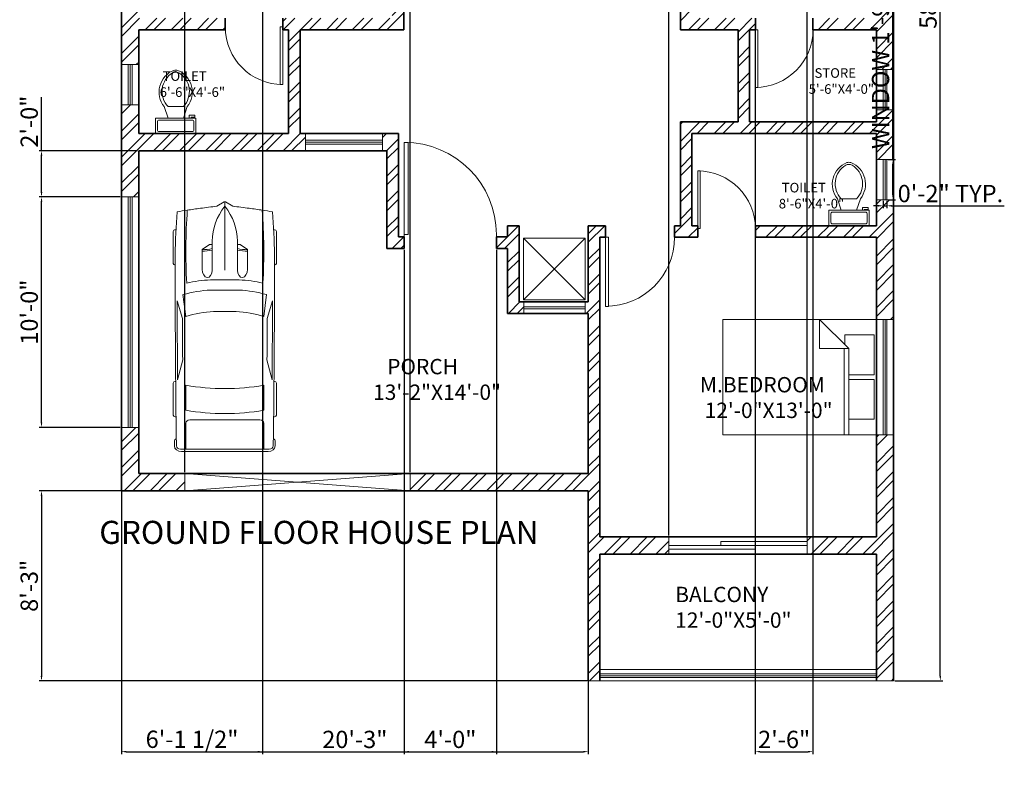
# Model space of a CAD drawing. Units: inches. Extents: x 73 to 724, y 1566 to 2355.
# Tile 1 of 2: x 147 to 660, y 1566 to 1955. Entities that reach past the tile are written whole.
import ezdxf

# ---------------------------------------------------------------- set-up
doc = ezdxf.new("R2010")
doc.units = ezdxf.units.IN
for name, color, linetype, lineweight in [('A-ANNO-DIMS', 2, 'Continuous', 18), ('A-ANNO-TEXT', 7, 'Continuous', 25), ('A-AREA-IDEN', 7, 'Continuous', 18), ('A-DOOR', 4, 'Continuous', 18), ('A-EQPM-VEHC', 8, 'Continuous', 13), ('A-FLOR', 7, 'Continuous', 18), ('A-FLOR-FIXT', 9, 'Continuous', 18), ('A-FLOR-RAIL', 244, 'Continuous', 18), ('A-FURN', 9, 'Continuous', 18), ('A-GLAZ', 244, 'Continuous', 18), ('A-WALL', 7, 'Continuous', 35), ('A-WALL-PATT', 252, 'Continuous', 13)]:
    doc.layers.add(name, color=color, linetype=linetype, lineweight=lineweight)
doc.styles.get("Standard").update_dxf_attribs({"font": 'arial.ttf'})
doc.dimstyles.new('ISO-25', dxfattribs={"dimtxt": 9, "dimasz": 2.5, "dimexe": 1.25, "dimexo": 0.625, "dimtad": 1, "dimlunit": 3, "dimtxsty": 'Standard', "dimcen": 2.5, "dimadec": 0, "dimazin": 0, "dimtfac": 1, "dimtmove": 0, "dimatfit": 3, "dimfxl": 1, "dimarcsym": 0})

# ---------------------------------------------------------------- blocks, each defined once
blk = doc.blocks.new('*U2')
for p, q in [((0, 0), (0, -6)), ((40, 0), (40, -6))]:
    blk.add_line(p, q)
blk.add_lwpolyline([(0, 0), (0, 40), (1.75, 40), (1.75, 0)], close=True)
blk.add_arc((0, 0), 40, 0, 90)
blk = doc.blocks.new('*U6')
for p, q in [((0, 0), (0, 6)), ((40, 0), (40, 6))]:
    blk.add_line(p, q)
blk.add_lwpolyline([(0, 0), (0, -40), (1.75, -40), (1.75, 0)], close=True)
blk.add_arc((0, 0), 40, 270, 0)
blk = doc.blocks.new('*U7')
for p, q in [((0, 0), (0, -6)), ((40, 0), (40, -6))]:
    blk.add_line(p, q)
blk.add_lwpolyline([(0, 0), (0, 40), (1.75, 40), (1.75, 0)], close=True)
blk.add_arc((0, 0), 40, 0, 90)
blk = doc.blocks.new('*U8')
for p, q in [((-40, 0), (-40, 6)), ((0, 0), (0, 6))]:
    blk.add_line(p, q)
blk.add_lwpolyline([(0, 0), (0, -40), (-1.75, -40), (-1.75, 0)], close=True)
blk.add_arc((0, 0), 40, 180, 270)
blk = doc.blocks.new('*D10')
at = {"layer": 'A-ANNO-DIMS', "color": 0, "lineweight": -2, "transparency": 16777216}
for p, q in [((602.66, 2307.12), (627.57, 2307.12)), ((626.32, 1613.62), (626.32, 2304.62)), ((602.66, 1611.12), (627.57, 1611.12))]:
    blk.add_line(p, q, dxfattribs=at)
at = {"layer": 'A-ANNO-DIMS', "color": 0, "transparency": 16777216}
for points in [[(625.9, 2304.62), (626.74, 2304.62), (626.32, 2307.12)], [(625.9, 1613.62), (626.74, 1613.62), (626.32, 1611.12)]]:
    blk.add_solid(points, dxfattribs=at)
at = {"layer": 'Defpoints', "color": 0, "transparency": 16777216}
for p in [(602.03, 2307.12), (626.32, 2307.12), (602.03, 1611.12)]:
    blk.add_point(p, dxfattribs=at)
at = {"layer": 'A-ANNO-DIMS', "color": 0, "transparency": 16777216, "insert": (621.1, 1959.12), "char_height": 9, "attachment_point": 5, "rotation": 90}
blk.add_mtext("58'", dxfattribs=at)
blk = doc.blocks.new('Bed - Queen')
for p, q in [((0, -80.00003), (0, 0)), ((0, 0), (59.99999, 0)), ((59.99999, 0), (59.99999, -80.00003)), ((7.99999, -1.2), (28.79998, -1.2)), ((7.99999, -14.4), (7.99999, -1.2)), ((28.79998, -1.2), (28.79998, -14.4)), ((31.19999, -1.2), (51.99999, -1.2)), ((31.19999, -14.4), (31.19999, -1.2)), ((51.99999, -1.2), (51.99999, -16.4)), ((0, -14.4), (44.8, -14.4)), ((59.99999, -29.6), (44.8, -14.4)), ((44.8, -14.4), (44.8, -29.6)), ((44.8, -16.8), (0, -16.8)), ((51.99999, -16.4), (46.79936, -16.4)), ((44.8, -29.6), (59.99999, -29.6)), ((59.99999, -80.00003), (0, -80.00003))]:
    blk.add_line(p, q)
blk = doc.blocks.new('*U13')
for p, q in [((9.5, -6), (9.5, -2)), ((-10, -8.5), (-8, -8.5)), ((-10, -9.5), (-10, -8.5)), ((-7, -9.5), (-10, -9.5)), ((-8, -8.5), (-8, -8)), ((-7, -8), (-7, -9.5)), ((-4, -8), (-6, -14)), ((4, -8), (6, -14)), ((4, -14), (-4, -14))]:
    blk.add_line(p, q)
blk.add_lwpolyline([(10.5, -8), (10.5, 0), (-10.5, 0), (-10.5, -8)], close=True)
for points in [[(-9.5, -2), (-9.5, -6)], [(8.5, -1), (-8.5, -1)], [(-8.5, -7), (8.5, -7)]]:
    blk.add_lwpolyline(points)
for centre, radius, start, end in [((-8.62, -1.88), 0.884, 81.8699, 188.1301), ((8.62, -1.88), 0.884, 351.8699, 98.1301), ((-8.62, -6.12), 0.884, 171.8699, 278.1301), ((8.62, -6.12), 0.884, 261.8699, 8.1301), ((3.52, -21.58), 12.17, 141.4691, 247.9714), ((4.2, -21.82), 11.33, 136.3677, 238.9468), ((-3.52, -21.58), 12.17, 292.0284, 38.5307), ((-4.2, -21.82), 11.33, 301.053, 43.6321), ((0, -27.88), 4, 245.7318, 294.2682), ((0, -29), 4, 254.8605, 285.1395)]:
    blk.add_arc(centre, radius, start, end)
blk = doc.blocks.new('*U15')
for p, q in [((21.1, 37.41), (21.1, 36.83)), ((46.55, 38.89), (22.35, 38.89)), ((47.8, 37.39), (47.8, 37.41)), ((135.45, 37.07), (135.45, 37.41)), ((136.7, 38.89), (160.9, 38.89)), ((162.15, 37.41), (162.15, 36.77)), ((70.03, 31.54), (86.41, 29.35)), ((87.99, 31.87), (74.76, 35.92)), ((134.31, 35.6), (119.29, 31.78)), ((186.47, -33.5), (186.47, 33.5)), ((188.4, -32.76), (188.4, 32.76)), ((138.42, 29.35), (157.25, 29.35)), ((164.52, 26.39), (164.52, -26.39)), ((186.47, 29.35), (167.01, 29.35)), ((32.27, 11.63), (36.13, 17.17)), ((36.13, 17.17), (50.94, 17.17)), ((29.77, 9.51), (51.68, 9.51)), ((32.12, 9.51), (32.12, 11.15)), ((58.92, -10.77), (58.92, 10.77)), ((66.55, -10.53), (66.55, 10.53)), ((82.74, 8.5), (82.74, -8.5)), ((186.47, -10.53), (186.47, 10.53)), ((3.27, 6.13), (0.1, 0.41)), ((0, 0), (51.68, 0)), ((0.1, -0.41), (3.27, -6.13)), ((29.77, -9.51), (51.68, -9.51)), ((32.12, -9.51), (32.12, -11.15)), ((32.27, -11.63), (36.13, -17.17)), ((36.13, -17.17), (50.94, -17.17)), ((86.41, -29.35), (70.03, -31.54)), ((157.25, -29.35), (138.42, -29.35)), ((167.01, -29.35), (186.47, -29.35)), ((21.1, -37.41), (21.1, -36.83)), ((87.99, -31.87), (74.76, -35.92)), ((134.31, -35.6), (119.29, -31.78)), ((135.45, -37.07), (135.45, -37.41)), ((162.15, -37.41), (162.15, -36.77)), ((46.55, -38.89), (22.35, -38.89)), ((47.8, -37.39), (47.8, -37.41)), ((136.7, -38.89), (160.9, -38.89))]:
    blk.add_line(p, q)
for centre, major_axis, ratio, start_param, end_param in [((41.19, -490.86), (0, 528.23), 0.842304, 0.00281, 0.075598), ((22.35, 37.41), (0, -1.48), 0.842304, 3.141593, 4.712389), ((64.48, -10555.62), (0, 10593.03), 0.842304, -0.013397, 0.002797), ((46.55, 37.41), (0, 1.48), 0.842304, -1.570796, 0), ((136.7, 37.41), (0, -1.48), 0.842304, 3.141593, 4.712389), ((160.9, 37.41), (0, 1.48), 0.842304, -1.570796, 0), ((180.63, 35.84), (0, 2.22), 0.842304, -0.013017, 1.249894), ((64.48, -10556.36), (0, 10595.31), 0.842304, -0.013397, -0.013017), ((183.98, 32.76), (0, -5.25), 0.842304, 1.570796, 3.128196), ((266.03, -27.52), (0, 313.31), 0.842304, 1.367076, 1.39176), ((37.47, -593.96), (0, -623.33), 0.842304, 3.096046, 3.200911), ((135.29, 5.39), (0, 81.77), 0.842304, 1.245306, 1.50788), ((64.48, -10555.62), (0, -10591.55), 0.842304, 3.133765, 3.140441), ((95.79, -3666.35), (0, -3698.24), 0.842304, 3.134049, 3.144098), ((183.98, 33.5), (0, -2.96), 0.842304, 1.570796, 3.128196), ((259.18, -27.52), (0, -305.3), 0.842304, 4.528606, 4.561838), ((134.4, 5.39), (0, -89.78), 0.842304, 4.449482, 4.652344), ((149.6, 2.8), (0, -79.58), 0.842304, 4.372215, 4.640744), ((17.08, 0), (0, 147.02), 0.842304, 4.511394, 4.913384), ((35.91, 0), (0, 147.02), 0.842304, 4.511394, 4.913384), ((167.01, 26.39), (0, 2.96), 0.842304, 0, 1.570796), ((-204.49, 52.4), (0, -250.96), 0.842304, 1.385369, 1.434372), ((13.04, 17.01), (0, 27.42), 0.842304, 4.435146, 4.718221), ((14.2, 17.01), (0, 27.42), 0.842304, 4.435146, 4.718221), ((50.79, 13.34), (6.34, -0.36), 0.603834, -1.395552, 1.581315), ((29.77, -46.66), (0, 56.17), 0.842304, 0, 0.590319), ((32.75, 11.15), (0, 0.74), 0.842304, 0.879714, 1.570796), ((0.62, 0), (0, -0.74), 0.842304, 4.131459, 5.293319), ((-204.49, -52.4), (0, 250.96), 0.842304, -1.434372, -1.385369), ((29.77, 46.66), (0, 56.17), 0.842304, 2.551274, 3.141593), ((32.75, -11.15), (0, -0.74), 0.842304, 4.712389, 5.403472), ((13.04, -17.01), (0, -27.42), 0.842304, 1.564964, 1.848039), ((14.2, -17.01), (0, -27.42), 0.842304, 1.564964, 1.848039), ((134.4, -5.39), (0, -89.78), 0.842304, -1.510751, -1.307889), ((135.29, -5.39), (0, -81.77), 0.842304, -1.50788, -1.245306), ((149.6, -2.8), (0, -79.58), 0.842304, -1.499151, -1.230623), ((259.18, 27.52), (0, 305.3), 0.842304, 1.721348, 1.754579), ((266.03, 27.52), (0, 313.31), 0.842304, 1.749832, 1.774517), ((37.47, 593.96), (0, -623.33), 0.842304, -0.059319, 0.045547), ((167.01, -26.39), (0, -2.96), 0.842304, 4.712389, 6.283185), ((41.19, 490.86), (0, -528.23), 0.842304, -0.075598, -0.00281), ((64.48, 10555.62), (0, 10593.03), 0.842304, 3.138796, 3.15499), ((64.48, 10555.62), (0, -10591.55), 0.842304, 0.001152, 0.007828), ((95.79, 3666.35), (0, -3698.24), 0.842304, -0.002505, 0.007544), ((180.63, -35.84), (0, -2.22), 0.842304, -1.249894, 0.013017), ((183.98, -33.5), (0, 2.96), 0.842304, 3.15499, 4.712389), ((183.98, -32.76), (0, -5.25), 0.842304, 0.013397, 1.570796), ((22.35, -37.41), (0, 1.48), 0.842304, 1.570796, 3.141593), ((46.55, -37.41), (0, -1.48), 0.842304, 0, 1.570796), ((136.7, -37.41), (0, -1.48), 0.842304, -1.570796, 0), ((160.9, -37.41), (0, 1.48), 0.842304, 3.141593, 4.712389), ((64.48, 10556.36), (0, 10595.31), 0.842304, 3.15461, 3.15499)]:
    blk.add_ellipse(centre, major_axis=major_axis, ratio=ratio, start_param=start_param, end_param=end_param)
at = {"extrusion": (0, 0, -1)}
blk.add_ellipse((50.79, -13.34), major_axis=(6.34, 0.36), ratio=0.603834, start_param=-1.395552, end_param=1.581315, dxfattribs=at)
blk = doc.blocks.new('WIN-GLAZING-60IN')
for p, q in [((0, 2), (60, 2)), ((0, 1), (60, 1)), ((0, 0), (60, 0))]:
    blk.add_line(p, q)
blk = doc.blocks.new('WIN-GLAZING-21IN')
for p, q in [((0, 21), (0, 0)), ((1, 21), (1, 0)), ((2, 21), (2, 0))]:
    blk.add_line(p, q)
blk = doc.blocks.new('*D21')
at = {"layer": 'A-ANNO-DIMS', "color": 0, "lineweight": -2, "transparency": 16777216}
for p, q in [((601.68, 1882.62), (601.68, 2000.26)), ((599.16, 1882.62), (602.93, 1882.62)), ((601.68, 1864.12), (601.68, 1880.12)), ((599.16, 1861.62), (602.93, 1861.62))]:
    blk.add_line(p, q, dxfattribs=at)
at = {"layer": 'A-ANNO-DIMS', "color": 0, "transparency": 16777216}
for points in [[(601.27, 1880.12), (602.1, 1880.12), (601.68, 1882.62)], [(601.27, 1864.12), (602.1, 1864.12), (601.68, 1861.62)]]:
    blk.add_solid(points, dxfattribs=at)
at = {"layer": 'Defpoints', "color": 0, "transparency": 16777216}
for p in [(598.53, 1882.62), (601.68, 1882.62), (598.53, 1861.62)]:
    blk.add_point(p, dxfattribs=at)
at = {"layer": 'A-ANNO-DIMS', "color": 0, "transparency": 16777216, "insert": (596.4, 1942.69), "char_height": 9, "attachment_point": 5, "rotation": 90}
blk.add_mtext('WINDOW 1\'-9" TYP.', dxfattribs=at)
blk = doc.blocks.new('*D22')
at = {"layer": 'A-ANNO-DIMS', "color": 0, "lineweight": -2, "transparency": 16777216}
for p, q in [((596.53, 1861), (596.53, 1857.22)), ((598.53, 1861), (598.53, 1857.22)), ((594.03, 1858.47), (591.53, 1858.47)), ((596.53, 1858.47), (598.53, 1858.47)), ((601.03, 1858.47), (659.64, 1858.47))]:
    blk.add_line(p, q, dxfattribs=at)
at = {"layer": 'A-ANNO-DIMS', "color": 0, "transparency": 16777216}
for points in [[(594.03, 1858.89), (594.03, 1858.06), (596.53, 1858.47)], [(601.03, 1858.89), (601.03, 1858.06), (598.53, 1858.47)]]:
    blk.add_solid(points, dxfattribs=at)
at = {"layer": 'Defpoints', "color": 0, "transparency": 16777216}
for p in [(596.53, 1861.62), (598.53, 1861.62), (598.53, 1858.47)]:
    blk.add_point(p, dxfattribs=at)
at = {"layer": 'A-ANNO-DIMS', "color": 0, "transparency": 16777216, "insert": (631.59, 1863.69), "char_height": 9, "attachment_point": 5}
blk.add_mtext('0\'-2" TYP.', dxfattribs=at)
blk = doc.blocks.new('*D27')
at = {"layer": 'A-ANNO-DIMS', "color": 0, "lineweight": -2, "transparency": 16777216}
for p, q in [((200.03, 1709.5), (200.03, 1573.02)), ((443.03, 1709.5), (443.03, 1573.02)), ((202.53, 1574.27), (440.53, 1574.27))]:
    blk.add_line(p, q, dxfattribs=at)
at = {"layer": 'A-ANNO-DIMS', "color": 0, "transparency": 16777216}
for points in [[(202.53, 1574.69), (202.53, 1573.86), (200.03, 1574.27)], [(440.53, 1574.69), (440.53, 1573.86), (443.03, 1574.27)]]:
    blk.add_solid(points, dxfattribs=at)
at = {"layer": 'Defpoints', "color": 0, "transparency": 16777216}
for p in [(200.03, 1710.12), (443.03, 1710.12), (443.03, 1574.27)]:
    blk.add_point(p, dxfattribs=at)
at = {"layer": 'A-ANNO-DIMS', "color": 0, "transparency": 16777216, "insert": (321.53, 1579.49), "char_height": 9, "attachment_point": 5}
blk.add_mtext('20\'-3"', dxfattribs=at)
blk = doc.blocks.new('*D28')
at = {"layer": 'A-ANNO-DIMS', "color": 0, "lineweight": -2, "transparency": 16777216}
for p, q in [((442.41, 1710.12), (157.17, 1710.12)), ((158.42, 1707.62), (158.42, 1613.62)), ((442.41, 1611.12), (157.17, 1611.12))]:
    blk.add_line(p, q, dxfattribs=at)
at = {"layer": 'A-ANNO-DIMS', "color": 0, "transparency": 16777216}
for points in [[(158, 1707.62), (158.84, 1707.62), (158.42, 1710.12)], [(158, 1613.62), (158.84, 1613.62), (158.42, 1611.12)]]:
    blk.add_solid(points, dxfattribs=at)
at = {"layer": 'Defpoints', "color": 0, "transparency": 16777216}
for p in [(443.03, 1710.12), (158.42, 1611.12), (443.03, 1611.12)]:
    blk.add_point(p, dxfattribs=at)
at = {"layer": 'A-ANNO-DIMS', "color": 0, "transparency": 16777216, "insert": (153.2, 1660.62), "char_height": 9, "attachment_point": 5, "rotation": 90}
blk.add_mtext('8\'-3"', dxfattribs=at)
blk = doc.blocks.new('*D31')
at = {"layer": 'A-ANNO-DIMS', "color": 0, "lineweight": -2, "transparency": 16777216}
for p, q in [((158.42, 1887.12), (158.42, 1914.95)), ((208.41, 1887.12), (157.17, 1887.12)), ((158.42, 1865.62), (158.42, 1884.62)), ((199.41, 1863.12), (157.17, 1863.12))]:
    blk.add_line(p, q, dxfattribs=at)
at = {"layer": 'A-ANNO-DIMS', "color": 0, "transparency": 16777216}
for points in [[(158, 1884.62), (158.84, 1884.62), (158.42, 1887.12)], [(158, 1865.62), (158.84, 1865.62), (158.42, 1863.12)]]:
    blk.add_solid(points, dxfattribs=at)
at = {"layer": 'Defpoints', "color": 0, "transparency": 16777216}
for p in [(158.42, 1887.12), (209.03, 1887.12), (200.03, 1863.12)]:
    blk.add_point(p, dxfattribs=at)
at = {"layer": 'A-ANNO-DIMS', "color": 0, "transparency": 16777216, "insert": (153.2, 1902.29), "char_height": 9, "attachment_point": 5, "rotation": 90}
blk.add_mtext('2\'-0"', dxfattribs=at)
blk = doc.blocks.new('*D35')
at = {"layer": 'A-ANNO-DIMS', "color": 0, "lineweight": -2, "transparency": 16777216}
for p, q in [((347.27, 1835.63), (347.27, 1573.02)), ((395.27, 1835.63), (395.27, 1573.02)), ((349.77, 1574.27), (392.77, 1574.27))]:
    blk.add_line(p, q, dxfattribs=at)
at = {"layer": 'A-ANNO-DIMS', "color": 0, "transparency": 16777216}
for points in [[(349.77, 1574.69), (349.77, 1573.86), (347.27, 1574.27)], [(392.77, 1574.69), (392.77, 1573.86), (395.27, 1574.27)]]:
    blk.add_solid(points, dxfattribs=at)
at = {"layer": 'Defpoints', "color": 0, "transparency": 16777216}
for p in [(347.27, 1836.26), (395.27, 1836.26), (395.27, 1574.27)]:
    blk.add_point(p, dxfattribs=at)
at = {"layer": 'A-ANNO-DIMS', "color": 0, "transparency": 16777216, "insert": (371.27, 1579.49), "char_height": 9, "attachment_point": 5}
blk.add_mtext('4\'-0"', dxfattribs=at)
blk = doc.blocks.new('*D36')
at = {"layer": 'A-ANNO-DIMS', "color": 0, "lineweight": -2, "transparency": 16777216}
for p, q in [((233.03, 1719.75), (233.03, 2345.22)), ((235.53, 2343.97), (347.77, 2343.97)), ((350.27, 1719.75), (350.27, 2345.22))]:
    blk.add_line(p, q, dxfattribs=at)
at = {"layer": 'A-ANNO-DIMS', "color": 0, "transparency": 16777216}
for points in [[(235.53, 2344.39), (235.53, 2343.56), (233.03, 2343.97)], [(347.77, 2344.39), (347.77, 2343.56), (350.27, 2343.97)]]:
    blk.add_solid(points, dxfattribs=at)
at = {"layer": 'Defpoints', "color": 0, "transparency": 16777216}
for p in [(350.27, 2343.97), (233.03, 1719.12), (350.27, 1719.12)]:
    blk.add_point(p, dxfattribs=at)
at = {"layer": 'A-ANNO-DIMS', "color": 0, "transparency": 16777216, "insert": (291.65, 2349.19), "char_height": 9, "attachment_point": 5}
blk.add_mtext('9\'-9"', dxfattribs=at)
blk = doc.blocks.new('*D37')
at = {"layer": 'A-ANNO-DIMS', "color": 0, "lineweight": -2, "transparency": 16777216}
for p, q in [((200.03, 1710.75), (200.03, 2345.22)), ((202.53, 2343.97), (230.53, 2343.97)), ((233.03, 1719.75), (233.03, 2345.22))]:
    blk.add_line(p, q, dxfattribs=at)
at = {"layer": 'A-ANNO-DIMS', "color": 0, "transparency": 16777216}
for points in [[(202.53, 2344.39), (202.53, 2343.56), (200.03, 2343.97)], [(230.53, 2344.39), (230.53, 2343.56), (233.03, 2343.97)]]:
    blk.add_solid(points, dxfattribs=at)
at = {"layer": 'Defpoints', "color": 0, "transparency": 16777216}
for p in [(233.03, 2343.97), (233.03, 1719.12), (200.03, 1710.12)]:
    blk.add_point(p, dxfattribs=at)
at = {"layer": 'A-ANNO-DIMS', "color": 0, "transparency": 16777216, "insert": (216.53, 2349.19), "char_height": 9, "attachment_point": 5}
blk.add_mtext('2\'-9"', dxfattribs=at)
blk = doc.blocks.new('*D38')
at = {"layer": 'A-ANNO-DIMS', "color": 0, "lineweight": -2, "transparency": 16777216}
for p, q in [((200.03, 2306.5), (200.03, 1573.02)), ((273.53, 2306.5), (273.53, 1573.02)), ((202.53, 1574.27), (271.03, 1574.27))]:
    blk.add_line(p, q, dxfattribs=at)
at = {"layer": 'A-ANNO-DIMS', "color": 0, "transparency": 16777216}
for points in [[(202.53, 1574.69), (202.53, 1573.86), (200.03, 1574.27)], [(271.03, 1574.69), (271.03, 1573.86), (273.53, 1574.27)]]:
    blk.add_solid(points, dxfattribs=at)
at = {"layer": 'Defpoints', "color": 0, "transparency": 16777216}
for p in [(200.03, 2307.12), (273.53, 2307.12), (273.53, 1574.27)]:
    blk.add_point(p, dxfattribs=at)
at = {"layer": 'A-ANNO-DIMS', "color": 0, "transparency": 16777216, "insert": (236.78, 1579.55), "char_height": 9, "attachment_point": 5}
blk.add_mtext('6\'-1 1/2"', dxfattribs=at)
blk = doc.blocks.new('*D40')
at = {"layer": 'A-ANNO-DIMS', "color": 0, "lineweight": -2, "transparency": 16777216}
for p, q in [((530.03, 1949.5), (530.03, 1573.02)), ((560.03, 1949.5), (560.03, 1573.02)), ((532.53, 1574.27), (557.53, 1574.27))]:
    blk.add_line(p, q, dxfattribs=at)
at = {"layer": 'A-ANNO-DIMS', "color": 0, "transparency": 16777216}
for points in [[(532.53, 1574.69), (532.53, 1573.86), (530.03, 1574.27)], [(557.53, 1574.69), (557.53, 1573.86), (560.03, 1574.27)]]:
    blk.add_solid(points, dxfattribs=at)
at = {"layer": 'Defpoints', "color": 0, "transparency": 16777216}
for p in [(530.03, 1950.12), (560.03, 1950.12), (560.03, 1574.27)]:
    blk.add_point(p, dxfattribs=at)
at = {"layer": 'A-ANNO-DIMS', "color": 0, "transparency": 16777216, "insert": (545.03, 1579.49), "char_height": 9, "attachment_point": 5}
blk.add_mtext('2\'-6"', dxfattribs=at)
blk = doc.blocks.new('*D45')
at = {"layer": 'A-ANNO-DIMS', "color": 0, "lineweight": -2, "transparency": 16777216}
for p, q in [((199.41, 1863.12), (157.17, 1863.12)), ((158.42, 1745.62), (158.42, 1860.62)), ((199.41, 1743.12), (157.17, 1743.12))]:
    blk.add_line(p, q, dxfattribs=at)
at = {"layer": 'A-ANNO-DIMS', "color": 0, "transparency": 16777216}
for points in [[(158, 1860.62), (158.84, 1860.62), (158.42, 1863.12)], [(158, 1745.62), (158.84, 1745.62), (158.42, 1743.12)]]:
    blk.add_solid(points, dxfattribs=at)
at = {"layer": 'Defpoints', "color": 0, "transparency": 16777216}
for p in [(158.42, 1863.12), (200.03, 1863.12), (200.03, 1743.12)]:
    blk.add_point(p, dxfattribs=at)
at = {"layer": 'A-ANNO-DIMS', "color": 0, "transparency": 16777216, "insert": (153.2, 1803.12), "char_height": 9, "attachment_point": 5, "rotation": 90}
blk.add_mtext('10\'-0"', dxfattribs=at)
blk = doc.blocks.new('*D46')
at = {"layer": 'A-ANNO-DIMS', "color": 0, "lineweight": -2, "transparency": 16777216}
for p, q in [((485.03, 1686.75), (485.03, 2345.22)), ((487.53, 2343.97), (554.53, 2343.97)), ((557.03, 1686.75), (557.03, 2345.22))]:
    blk.add_line(p, q, dxfattribs=at)
at = {"layer": 'A-ANNO-DIMS', "color": 0, "transparency": 16777216}
for points in [[(487.53, 2344.39), (487.53, 2343.56), (485.03, 2343.97)], [(554.53, 2344.39), (554.53, 2343.56), (557.03, 2343.97)]]:
    blk.add_solid(points, dxfattribs=at)
at = {"layer": 'Defpoints', "color": 0, "transparency": 16777216}
for p in [(557.03, 2343.97), (485.03, 1686.12), (557.03, 1686.12)]:
    blk.add_point(p, dxfattribs=at)
at = {"layer": 'A-ANNO-DIMS', "color": 0, "transparency": 16777216, "insert": (521.03, 2349.19), "char_height": 9, "attachment_point": 5}
blk.add_mtext('6\'-0"', dxfattribs=at)

msp = doc.modelspace()

# ---------------------------------------------------------------- hatches: boundary and pattern name
at = {"layer": 'A-WALL-PATT'}
h = msp.add_hatch(dxfattribs=at)
h.set_pattern_fill('ANSI32', color=256)
h.paths.add_polyline_path([(209.035, 2088.122), (341.035, 2088.122), (341.035, 2085.122), (341.635, 2085.122), (347.035, 2085.122), (347.035, 2094.122), (293.035, 2094.122), (293.035, 2148.122), (359.035, 2148.122), (359.035, 2154.122), (284.035, 2154.122), (284.035, 2149.622), (284.035, 2148.122), (287.035, 2148.122), (287.035, 2094.122), (209.035, 2094.122), (209.035, 2109.443), (200.035, 2109.443), (200.035, 2052.122), (209.035, 2052.122)])
h.paths.add_polyline_path([(347.035, 2049.122), (341.035, 2049.122), (341.035, 1956.122), (284.035, 1956.122), (284.035, 1951.622), (284.035, 1950.122), (287.035, 1950.122), (287.035, 1896.122), (209.035, 1896.122), (209.035, 1910.964), (200.035, 1910.964), (200.035, 1863.122), (209.035, 1863.122), (209.035, 1887.122), (295.787, 1887.122), (295.787, 1896.122), (293.035, 1896.122), (293.035, 1950.122), (347.035, 1950.122)])
h.paths.add_polyline_path([(209.035, 1992.122), (200.035, 1992.122), (200.035, 1931.964), (209.035, 1931.964), (209.035, 1950.122), (254.035, 1950.122), (254.035, 1956.122), (209.035, 1956.122)], flags=17)
h.paths.add_polyline_path([(344.268, 1896.122), (335.891, 1896.122), (335.891, 1887.122), (338.268, 1887.122), (338.268, 1836.258), (347.268, 1836.258), (347.268, 1842.258), (344.268, 1842.258)])
h.paths.add_polyline_path([(449.035, 1842.122), (452.035, 1842.122), (452.035, 1848.122), (443.035, 1848.122), (443.035, 1808.396), (441.494, 1808.396), (441.494, 1802.396), (443.035, 1802.396), (443.035, 1719.122), (350.268, 1719.122), (350.268, 1710.122), (443.035, 1710.122), (443.035, 1611.122), (449.035, 1611.122), (449.035, 1677.122), (485.035, 1677.122), (485.035, 1686.122), (449.035, 1686.122)])
h.paths.add_polyline_path([(407.035, 1848.122), (401.035, 1848.122), (401.035, 1842.258), (395.268, 1842.258), (395.268, 1836.258), (401.035, 1836.258), (401.035, 1802.396), (409.436, 1802.396), (409.436, 1808.396), (407.035, 1808.396)], flags=17)
h.paths.add_polyline_path([(497.035, 1896.122), (593.035, 1896.122), (593.035, 1882.622), (602.035, 1882.622), (602.035, 1908.472), (593.035, 1908.472), (593.035, 1902.122), (527.035, 1902.122), (527.035, 1950.122), (530.035, 1950.122), (530.035, 1956.122), (497.035, 1956.122), (497.035, 1968.122), (491.035, 1968.122), (491.035, 1950.122), (521.035, 1950.122), (521.035, 1902.122), (491.035, 1902.122), (491.035, 1848.122), (488.035, 1848.122), (488.035, 1842.122), (500.035, 1842.122), (500.035, 1848.122), (497.035, 1848.122)])
h.paths.add_polyline_path([(602.035, 1861.622), (593.035, 1861.622), (593.035, 1848.122), (530.035, 1848.122), (530.035, 1842.122), (593.035, 1842.122), (593.035, 1799.304), (602.035, 1799.304)])
h.paths.add_polyline_path([(602.035, 1739.304), (593.035, 1739.304), (593.035, 1686.122), (557.035, 1686.122), (557.035, 1677.122), (593.035, 1677.122), (593.035, 1611.122), (602.035, 1611.122)])
h.paths.add_polyline_path([(209.035, 1743.122), (200.035, 1743.122), (200.035, 1710.122), (233.035, 1710.122), (233.035, 1719.122), (209.035, 1719.122)])
h.paths.add_polyline_path([(602.035, 1996.783), (593.035, 1996.783), (593.035, 1956.122), (560.035, 1956.122), (560.035, 1950.122), (593.035, 1950.122), (593.035, 1929.472), (602.035, 1929.472)])
h.paths.add_polyline_path([(602.035, 2097.565), (593.035, 2097.565), (593.035, 2094.122), (515.035, 2094.122), (515.035, 2148.122), (518.035, 2148.122), (518.035, 2154.122), (443.035, 2154.122), (443.035, 2148.122), (509.035, 2148.122), (509.035, 2094.122), (491.035, 2094.122), (491.035, 2004.122), (497.035, 2004.122), (497.035, 2088.122), (593.035, 2088.122), (593.035, 2056.783), (602.035, 2056.783)])
h.paths.add_polyline_path([(602.035, 2196.587), (593.035, 2196.587), (593.035, 2154.122), (548.035, 2154.122), (548.035, 2148.122), (593.035, 2148.122), (593.035, 2118.565), (602.035, 2118.565)])
h.paths.add_polyline_path([(602.035, 2307.122), (528.535, 2307.122), (528.535, 2298.122), (593.035, 2298.122), (593.035, 2256.587), (602.035, 2256.587)])
h.paths.add_polyline_path([(468.535, 2307.122), (333.535, 2307.122), (333.535, 2298.122), (398.035, 2298.122), (398.035, 2154.122), (395.035, 2154.122), (395.035, 2148.122), (407.035, 2148.122), (407.035, 2154.122), (404.035, 2154.122), (404.035, 2298.122), (468.535, 2298.122)])
h.paths.add_polyline_path([(273.535, 2307.122), (200.035, 2307.122), (200.035, 2256.122), (209.035, 2256.122), (209.035, 2298.122), (273.535, 2298.122)])
h.paths.add_polyline_path([(209.035, 2196.122), (200.035, 2196.122), (200.035, 2130.443), (209.035, 2130.443), (209.035, 2148.122), (254.035, 2148.122), (254.035, 2154.122), (209.035, 2154.122)])

# ---------------------------------------------------------------- linework, layer by layer
at = {"layer": 'A-DOOR'}
for p, q in [((233.035, 1719.122), (233.035, 1710.122)), ((233.035, 1710.122), (350.268, 1719.122)), ((350.268, 1710.122), (233.035, 1719.122)), ((350.268, 1710.122), (350.268, 1719.122)), ((485.035, 1677.122), (485.035, 1686.122)), ((485.035, 1681.622), (557.035, 1681.622)), ((512.035, 1683.622), (557.035, 1683.622)), ((512.035, 1681.622), (512.035, 1683.622)), ((530.035, 1681.622), (530.035, 1679.622)), ((557.035, 1677.122), (557.035, 1686.122)), ((485.035, 1679.622), (530.035, 1679.622))]:
    msp.add_line(p, q, dxfattribs=at)
at = {"layer": 'A-FLOR'}
for p, q in [((409.291, 1841.569), (441.407, 1809.592)), ((409.291, 1809.592), (441.407, 1841.569))]:
    msp.add_line(p, q, dxfattribs=at)
msp.add_lwpolyline([(409.291, 1841.569), (441.407, 1841.569), (441.407, 1809.592), (409.291, 1809.592)], close=True, dxfattribs=at)
at = {"layer": 'A-FLOR-RAIL'}
for p, q in [((449.035, 1617.122), (593.035, 1617.122)), ((449.035, 1614.823), (593.035, 1614.823)), ((443.035, 1611.122), (602.035, 1611.122)), ((449.035, 1613.823), (593.035, 1613.823)), ((449.035, 1612.823), (593.035, 1612.823))]:
    msp.add_line(p, q, dxfattribs=at)
at = {"layer": 'A-GLAZ'}
for p, q in [((335.891, 1892.622), (295.787, 1892.622)), ((335.891, 1891.622), (295.787, 1891.622)), ((335.891, 1890.622), (295.787, 1890.622)), ((209.035, 1863.122), (200.035, 1863.122)), ((203.535, 1863.122), (203.535, 1743.122)), ((204.535, 1863.122), (204.535, 1743.122)), ((205.535, 1863.122), (205.535, 1743.122)), ((441.494, 1805.896), (409.436, 1805.896)), ((441.494, 1804.896), (409.436, 1804.896)), ((209.035, 1743.122), (200.035, 1743.122))]:
    msp.add_line(p, q, dxfattribs=at)
for points in [[(200.035, 1931.964), (209.035, 1931.964), (209.035, 1910.964), (200.035, 1910.964)], [(593.035, 1929.472), (602.035, 1929.472), (602.035, 1908.472), (593.035, 1908.472)], [(335.891, 1896.122), (335.891, 1887.122), (295.787, 1887.122), (295.787, 1896.122)], [(593.035, 1882.622), (602.035, 1882.622), (602.035, 1861.622), (593.035, 1861.622)], [(441.494, 1808.396), (441.494, 1802.396), (409.436, 1802.396), (409.436, 1808.396)], [(602.035, 1799.304), (602.035, 1739.304), (593.035, 1739.304), (593.035, 1799.304)]]:
    msp.add_lwpolyline(points, close=True, dxfattribs=at)
at = {"layer": 'A-WALL'}
for p, q in [((200.035, 2307.122), (200.035, 1710.122)), ((602.035, 2307.122), (602.035, 1611.122)), ((347.035, 2049.122), (347.035, 1950.122)), ((491.035, 1968.122), (491.035, 1950.122)), ((254.035, 1950.122), (254.035, 1956.122)), ((284.035, 1950.122), (284.035, 1956.122)), ((530.035, 1950.122), (530.035, 1956.122)), ((560.035, 1950.122), (560.035, 1956.122)), ((209.035, 1950.122), (254.035, 1950.122)), ((209.035, 1950.122), (209.035, 1896.122)), ((284.035, 1950.122), (287.035, 1950.122)), ((287.035, 1950.122), (287.035, 1896.122)), ((293.035, 1950.122), (293.035, 1896.122)), ((293.035, 1950.122), (347.035, 1950.122)), ((491.035, 1950.122), (521.035, 1950.122)), ((521.035, 1950.122), (521.035, 1902.122)), ((527.035, 1950.122), (527.035, 1902.122)), ((527.035, 1950.122), (530.035, 1950.122)), ((560.035, 1950.122), (593.035, 1950.122)), ((593.035, 1950.122), (593.035, 1902.122)), ((491.035, 1902.122), (521.035, 1902.122)), ((491.035, 1902.122), (491.035, 1848.122)), ((527.035, 1902.122), (593.035, 1902.122)), ((209.035, 1896.122), (287.035, 1896.122)), ((293.035, 1896.122), (344.268, 1896.122)), ((344.268, 1842.258), (344.268, 1896.122)), ((497.035, 1896.122), (593.035, 1896.122)), ((497.035, 1896.122), (497.035, 1848.122)), ((593.035, 1896.122), (593.035, 1848.122)), ((209.035, 1887.122), (338.268, 1887.122)), ((209.035, 1887.122), (209.035, 1719.122)), ((338.268, 1836.258), (338.268, 1887.122)), ((401.035, 1848.122), (407.035, 1848.122)), ((401.035, 1848.122), (401.035, 1842.258)), ((407.035, 1848.122), (407.035, 1808.396)), ((443.035, 1848.122), (443.035, 1808.396)), ((443.035, 1848.122), (452.035, 1848.122)), ((452.035, 1848.122), (452.035, 1842.122)), ((488.035, 1848.122), (488.035, 1842.122)), ((488.035, 1848.122), (491.035, 1848.122)), ((497.035, 1848.122), (500.035, 1848.122)), ((500.035, 1848.122), (500.035, 1842.122)), ((530.035, 1848.122), (530.035, 1842.122)), ((530.035, 1848.122), (593.035, 1848.122)), ((347.268, 1842.258), (344.268, 1842.258)), ((347.268, 1842.258), (347.268, 1836.258)), ((401.035, 1842.258), (395.268, 1842.258)), ((395.268, 1842.258), (395.268, 1836.258)), ((449.035, 1842.122), (452.035, 1842.122)), ((449.035, 1842.122), (449.035, 1686.122)), ((488.035, 1842.122), (500.035, 1842.122)), ((530.035, 1842.122), (593.035, 1842.122)), ((593.035, 1842.122), (593.035, 1686.122)), ((347.268, 1836.258), (338.268, 1836.258)), ((401.035, 1836.258), (395.268, 1836.258)), ((401.035, 1836.258), (401.035, 1802.396)), ((443.035, 1808.396), (407.035, 1808.396)), ((443.035, 1802.396), (401.035, 1802.396)), ((443.035, 1802.396), (443.035, 1719.122)), ((209.035, 1719.122), (443.035, 1719.122)), ((200.035, 1710.122), (443.035, 1710.122)), ((443.035, 1710.122), (443.035, 1611.122)), ((449.035, 1686.122), (593.035, 1686.122)), ((449.035, 1677.122), (593.035, 1677.122)), ((449.035, 1677.122), (449.035, 1611.122)), ((593.035, 1677.122), (593.035, 1611.122))]:
    msp.add_line(p, q, dxfattribs=at)

# ---------------------------------------------------------------- block references
at = {"layer": 'A-DOOR'}
for name, p, xscale, yscale, zscale in [('*U8', (284.035, 1951.622), 0.7500000000000026, 0.7500000000000026, 0.7500000000000026), ('*U6', (530.035, 1950.122), 0.7500000000000026, 0.7500000000000026, 0.7500000000000026), ('*U2', (347.268, 1843.458), 1.199999999999999, 1.199999999999999, 1.199999999999999), ('*U7', (500.035, 1846.622), 0.7500000000000026, 0.7500000000000026, 0.7500000000000026), ('*U6', (452.035, 1842.122), 0.9000000000000014, 0.9000000000000014, 0.9000000000000014)]:
    msp.add_blockref(name, p, dxfattribs=dict(at, xscale=xscale, yscale=yscale, zscale=zscale))
at = {"layer": 'A-EQPM-VEHC', "xscale": 0.6904173281838752, "yscale": 0.6904173281838752, "zscale": 0.6904173281838752, "rotation": 270}
msp.add_blockref('*U15', (253.855, 1860.584), dxfattribs=at)
at = {"layer": 'A-FLOR-FIXT', "rotation": 180}
for p in [(228.279, 1896.122), (578.754, 1848.122)]:
    msp.add_blockref('*U13', p, dxfattribs=at)
at = {"layer": 'A-FURN', "xscale": -1, "rotation": 270}
msp.add_blockref('Bed - Queen', (593.035, 1739.304), dxfattribs=at)
at = {"layer": 'A-GLAZ'}
for p in [(203.535, 1910.964), (596.535, 1908.472), (596.535, 1861.622)]:
    msp.add_blockref('WIN-GLAZING-21IN', p, dxfattribs=at)
at = {"layer": 'A-GLAZ', "rotation": 90.00000000000088}
msp.add_blockref('WIN-GLAZING-60IN', (598.534, 1739.304), dxfattribs=at)

# ---------------------------------------------------------------- texts
at = {"layer": 'A-ANNO-TEXT', "insert": (188.496, 1694.449), "char_height": 12, "attachment_point": 1}
msp.add_mtext_dynamic_manual_height_columns('GROUND FLOOR HOUSE PLAN', width=257.76953, gutter_width=12.5, heights=[0], dxfattribs=at)
at = {"layer": 'A-AREA-IDEN', "attachment_point": 1}
for s, width, insert, char_height in [(' TOILET\\P6\'-6"X4\'-6"', 32.10823, (219.934, 1928.505), 5), ('  STORE\\P5\'-6"X4\'-0"', 32.10823, (557.805, 1930.111), 5), (' TOILET\\P8\'-6"X4\'-0"', 32.10823, (542.244, 1870.441), 5), ('   PORCH\\P13\'-2"X14\'-0"', 62.47038, (331.038, 1778.752), 8), ('M.BEDROOM\\P 12\'-0"X13\'-0"', 75.3198, (501.199, 1769.323), 8), ('BALCONY 12\'-0"X5\'-0"', 56.61603, (488.314, 1660.119), 8)]:
    msp.add_mtext_dynamic_manual_height_columns(s, width=width, gutter_width=12.5, heights=[0], dxfattribs=dict(at, insert=insert, char_height=char_height))

# ---------------------------------------------------------------- dimensions: what is measured, and where the dimension line sits
at = {"layer": 'A-ANNO-DIMS'}
for base, p1, p2, picture, middle in [((233.035, 2343.972), (200.035, 1710.122), (233.035, 1719.122), '*D37', (216.535, 2349.192)), ((350.268, 2343.972), (233.035, 1719.122), (350.268, 1719.122), '*D36', (291.651, 2349.192)), ((557.035, 2343.972), (485.035, 1686.122), (557.035, 1686.122), '*D46', (521.035, 2349.192)), ((273.535, 1574.272), (200.035, 2307.122), (273.535, 2307.122), '*D38', (236.785, 1579.55)), ((560.035, 1574.272), (530.035, 1950.122), (560.035, 1950.122), '*D40', (545.035, 1579.492)), ((395.268, 1574.272), (347.268, 1836.258), (395.268, 1836.258), '*D35', (371.268, 1579.492)), ((443.035, 1574.272), (200.035, 1710.122), (443.035, 1710.122), '*D27', (321.535, 1579.495))]:
    dim = msp.add_linear_dim(base=base, p1=p1, p2=p2, dimstyle='ISO-25', override={"dimdec": 1, "dimlfac": 1, "dimrnd": 0, "dimzin": 1, "dimdsep": 46, "dimlunit": 4, "dimfrac": 2}, dxfattribs=at)
    dim.commit()
    dim.dimension.update_dxf_attribs({"geometry": picture, "text_midpoint": middle})
for base, p1, p2, override, picture, middle in [((626.32, 2307.122), (602.035, 1611.122), (602.035, 2307.122), {"dimclrd": 0, "dimclre": 0, "dimclrt": 0}, '*D10', (621.1, 1959.122)), ((158.42, 1887.122), (200.035, 1863.122), (209.035, 1887.122), {"dimdec": 1, "dimlfac": 1, "dimrnd": 0, "dimzin": 1, "dimdsep": 46, "dimlunit": 4, "dimfrac": 2}, '*D31', (153.2, 1902.286)), ((158.42, 1863.122), (200.035, 1743.122), (200.035, 1863.122), {"dimdec": 1, "dimlfac": 1, "dimrnd": 0, "dimzin": 1, "dimdsep": 46, "dimlunit": 4, "dimfrac": 2}, '*D45', (153.2, 1803.122)), ((158.42, 1611.122), (443.035, 1710.122), (443.035, 1611.122), {"dimdec": 1, "dimlfac": 1, "dimrnd": 0, "dimzin": 1, "dimdsep": 46, "dimlunit": 4, "dimfrac": 2}, '*D28', (153.197, 1660.622))]:
    dim = msp.add_linear_dim(base=base, p1=p1, p2=p2, angle=90, dimstyle='ISO-25', override=override, dxfattribs=at)
    dim.commit()
    dim.dimension.update_dxf_attribs({"geometry": picture, "text_midpoint": middle})
dim = msp.add_linear_dim(base=(601.685, 1882.622), p1=(598.535, 1861.622), p2=(598.535, 1882.622), angle=90, text='WINDOW <> TYP.', dimstyle='ISO-25', override={"dimdec": 1, "dimlfac": 1, "dimrnd": 0, "dimzin": 1, "dimdsep": 46, "dimlunit": 4, "dimfrac": 2}, dxfattribs=at)
dim.commit()
dim.dimension.update_dxf_attribs({"geometry": '*D21', "text_midpoint": (596.403, 1942.69)})
dim = msp.add_linear_dim(base=(598.535, 1858.472), p1=(596.535, 1861.622), p2=(598.535, 1861.622), text='<> TYP.', dimstyle='ISO-25', override={"dimdec": 1, "dimlfac": 1, "dimrnd": 0, "dimzin": 1, "dimdsep": 46, "dimlunit": 4, "dimfrac": 2}, dxfattribs=at)
dim.commit()
dim.dimension.update_dxf_attribs({"geometry": '*D22', "text_midpoint": (631.589, 1863.692)})

doc.saveas('drawing.dxf')
